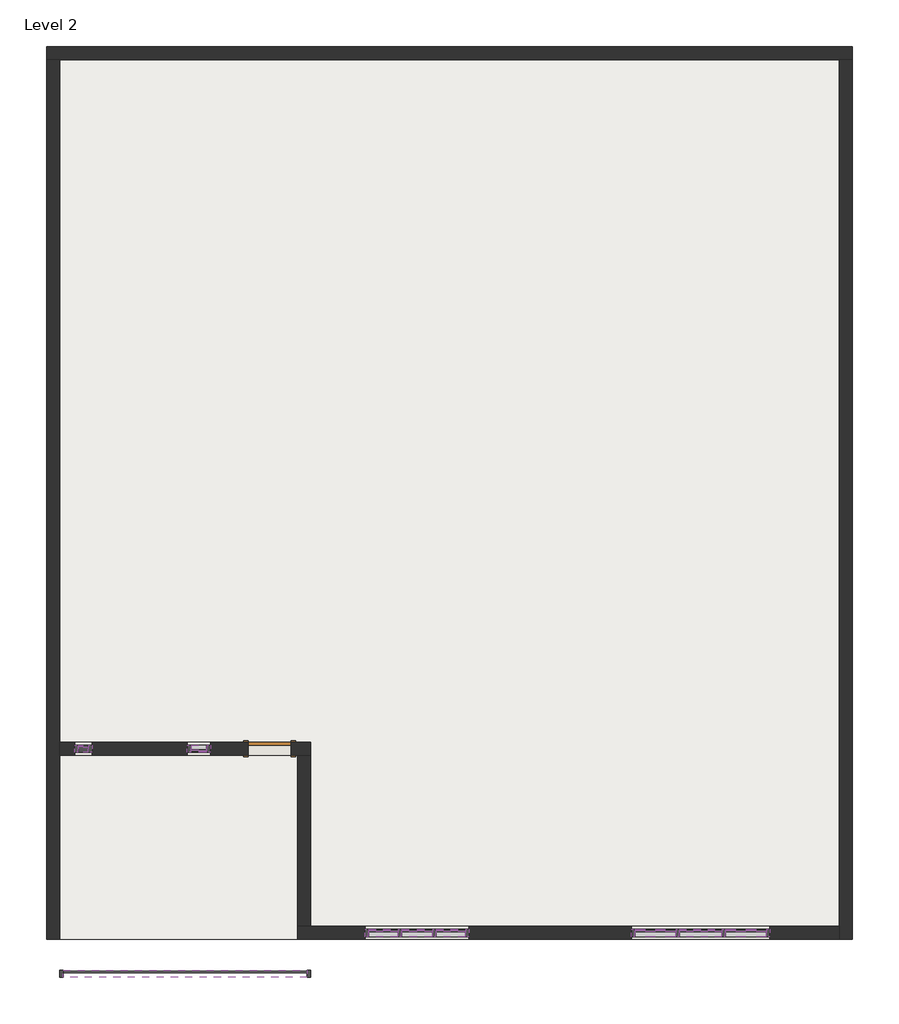
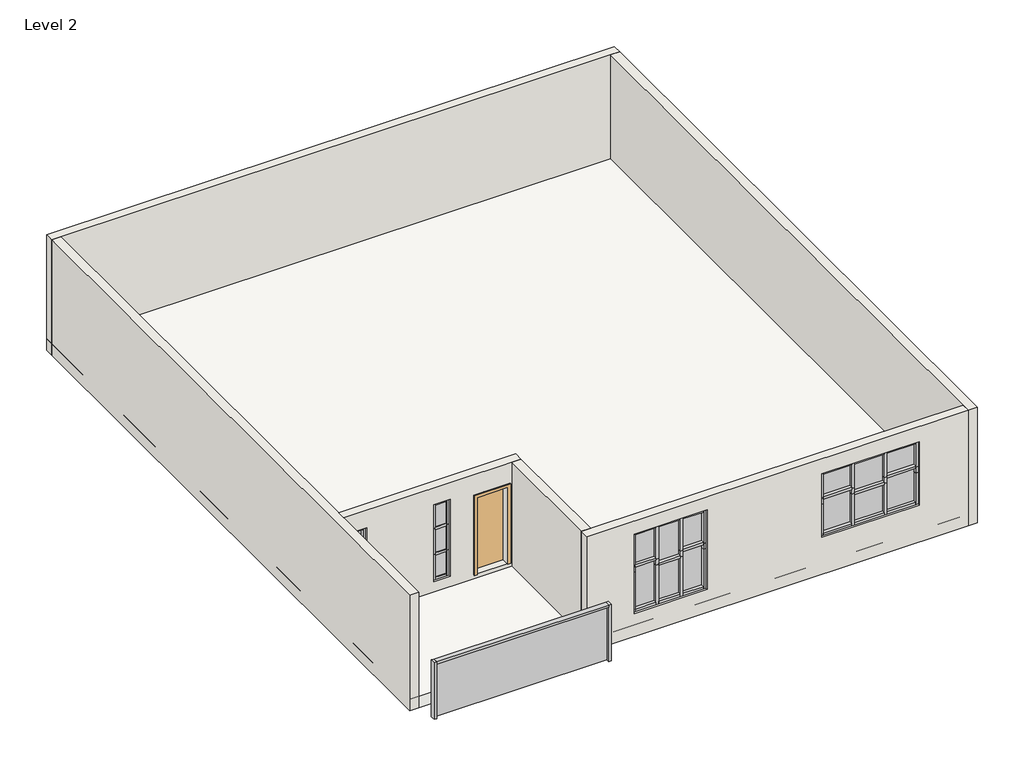
# One storey: 65 members, 19 plates, 6 walls, 1 door, 1 roof.
"""IFC4 building model written with IfcOpenShell, lengths in millimetres."""

from ifc_helpers import new_model, si_unit, frame, origin, place, context, project, spatial, polyline, outline, extrude, faceted_brep, transform, mapped, element, save
from components import door_a1484949, member_aaa03826, member_0b7646a3, member_a980948f, member_0a1a1ade, member_876f8f00, member_f6f0dfdd, member_50c8646f, member_e2125230, member_501daf10, member_2a6e7b3e, member_892f3d40, member_7007ad49, member_abeaf8ac, member_2c92067c, member_9d02be77, member_798d6cad, member_1bc815af, member_262c5f3f, member_6be37683, member_d3323a85, member_819a76f2, member_187b6476, member_d92184fb, member_2118ea0c, member_241584b0, member_4da692ab, system_panel_glazed_51e75bbe, system_panel_glazed_29e6fa37, system_panel_glazed_a0a4d195, system_panel_glazed_09326d9e, system_panel_glazed_ba8d0b35, system_panel_glazed_02566968, system_panel_glazed_4b08eeb4, system_panel_glazed_a2941881, system_panel_glazed_2307425d, system_panel_glazed_f1f3e2b8, system_panel_glazed_c39d0069, system_panel_glazed_879596d7, system_panel_glazed_4ec28fe5

model = new_model("IFC4")

# Units and contexts
model_context = context("Model", 3, world=origin())
ifc_project = project(units=[si_unit("LENGTHUNIT", "METRE", prefix="MILLI")], contexts=[model_context])

# Site, building, storey
site = spatial("IfcSite", under=ifc_project)
building = spatial("IfcBuilding", under=site)
storey = spatial("IfcBuildingStorey", under=building, Name="Level 2", Elevation=3048.0)

# Door
placement = place(None, origin())
door_shape = door_a1484949(model_context)
element("IfcDoor", 1, ObjectType="Single-Flush : 30\" x 80\"", at=placement, inside=storey, context=model_context, shape_type="MappedRepresentation", body=[
    mapped(door_shape, transform((-15264.8403308, -10002.5518738, 3454.4), x_axis=(1.0, 0.0, 0.0), y_axis=(0.0, 1.0, 0.0), z_axis=(0.0, 0.0, 1.0))),
])

# Members
member_shape = member_aaa03826(model_context)
element("IfcMember", 2, ObjectType="Rectangular Mullion : 2.5\" x 5\" rectangular", at=placement, inside=storey, context=model_context, shape_type="MappedRepresentation", body=[
    mapped(member_shape, transform((-11823.1403308, -13241.0518738, 4852.5078277), x_axis=(0.0, 0.0, 1.0), y_axis=(0.0, -1.0, 0.0), z_axis=(1.0, 0.0, 0.0))),
])
element("IfcMember", 3, ObjectType="Rectangular Mullion : 2.5\" x 5\" rectangular", at=placement, inside=storey, context=model_context, shape_type="MappedRepresentation", body=[
    mapped(member_shape, transform((-13010.5903308, -13241.0518738, 4852.5078277), x_axis=(0.0, 0.0, 1.0), y_axis=(0.0, -1.0, 0.0), z_axis=(1.0, 0.0, 0.0))),
])
member_2_shape = member_0b7646a3(model_context)
element("IfcMember", 4, ObjectType="Rectangular Mullion : 2.5\" x 5\" rectangular", at=placement, inside=storey, context=model_context, shape_type="MappedRepresentation", body=[
    mapped(member_2_shape, transform((-13010.5903308, -13241.0518738, 5747.4569224), x_axis=(0.0, 0.0, 1.0), y_axis=(0.0, -1.0, 0.0), z_axis=(1.0, 0.0, 0.0))),
])
element("IfcMember", 5, ObjectType="Rectangular Mullion : 2.5\" x 5\" rectangular", at=placement, inside=storey, context=model_context, shape_type="MappedRepresentation", body=[
    mapped(member_2_shape, transform((-11823.1403308, -13241.0518738, 5747.4569224), x_axis=(0.0, 0.0, 1.0), y_axis=(0.0, -1.0, 0.0), z_axis=(1.0, 0.0, 0.0))),
])
member_3_shape = member_a980948f(model_context)
element("IfcMember", 6, ObjectType="Rectangular Mullion : 2.5\" x 5\" rectangular", at=placement, inside=storey, context=model_context, shape_type="MappedRepresentation", body=[
    mapped(member_3_shape, transform((-12400.9903308, -13241.0518738, 5747.4569224), x_axis=(0.0, 0.0, 1.0), y_axis=(0.0, -1.0, 0.0), z_axis=(1.0, 0.0, 0.0))),
])
member_4_shape = member_0a1a1ade(model_context)
element("IfcMember", 7, ObjectType="Rectangular Mullion : 2.5\" x 5\" rectangular", at=placement, inside=storey, context=model_context, shape_type="MappedRepresentation", body=[
    mapped(member_4_shape, transform((-12400.9903308, -13241.0518738, 4700.1078277), x_axis=(0.0, 0.0, 1.0), y_axis=(0.0, -1.0, 0.0), z_axis=(1.0, 0.0, 0.0))),
])
element("IfcMember", 8, ObjectType="Rectangular Mullion : 2.5\" x 5\" rectangular", at=placement, inside=storey, context=model_context, shape_type="MappedRepresentation", body=[
    mapped(member_2_shape, transform((-12337.4903308, -13241.0518738, 3652.758733), x_axis=(0.0, 0.0, -1.0), y_axis=(0.0, -1.0, 0.0), z_axis=(-1.0, 0.0, 0.0))),
])
element("IfcMember", 9, ObjectType="Rectangular Mullion : 2.5\" x 5\" rectangular", at=placement, inside=storey, context=model_context, shape_type="MappedRepresentation", body=[
    mapped(member_2_shape, transform((-13524.9403308, -13241.0518738, 3652.758733), x_axis=(0.0, 0.0, -1.0), y_axis=(0.0, -1.0, 0.0), z_axis=(-1.0, 0.0, 0.0))),
])
element("IfcMember", 10, ObjectType="Rectangular Mullion : 2.5\" x 5\" rectangular", at=placement, inside=storey, context=model_context, shape_type="MappedRepresentation", body=[
    mapped(member_3_shape, transform((-12947.0903308, -13241.0518738, 3652.758733), x_axis=(0.0, 0.0, -1.0), y_axis=(0.0, -1.0, 0.0), z_axis=(-1.0, 0.0, 0.0))),
])
member_5_shape = member_876f8f00(model_context)
element("IfcMember", 11, ObjectType="Rectangular Mullion : 2.5\" x 5\" rectangular", at=placement, inside=storey, context=model_context, shape_type="MappedRepresentation", body=[
    mapped(member_5_shape, transform((-13588.4403308, -13241.0518738, 4852.5078277), x_axis=(-1.0, 0.0, 0.0), y_axis=(0.0, -1.0, 0.0), z_axis=(0.0, 0.0, 1.0))),
])
element("IfcMember", 12, ObjectType="Rectangular Mullion : 2.5\" x 5\" rectangular", at=placement, inside=storey, context=model_context, shape_type="MappedRepresentation", body=[
    mapped(member_5_shape, transform((-8902.1403308, -13241.0518738, 5010.2067568), x_axis=(-1.0, 0.0, 0.0), y_axis=(0.0, -1.0, 0.0), z_axis=(0.0, 0.0, 1.0))),
])
element("IfcMember", 13, ObjectType="Rectangular Mullion : 2.5\" x 5\" rectangular", at=placement, inside=storey, context=model_context, shape_type="MappedRepresentation", body=[
    mapped(member_5_shape, transform((-11759.6403308, -13241.0518738, 4700.1078277), x_axis=(1.0, 0.0, 0.0), y_axis=(0.0, -1.0, 0.0), z_axis=(0.0, 0.0, -1.0))),
])
element("IfcMember", 14, ObjectType="Rectangular Mullion : 2.5\" x 5\" rectangular", at=placement, inside=storey, context=model_context, shape_type="MappedRepresentation", body=[
    mapped(member_5_shape, transform((-6463.7403308, -13241.0518738, 4857.8067568), x_axis=(1.0, 0.0, 0.0), y_axis=(0.0, -1.0, 0.0), z_axis=(0.0, 0.0, -1.0))),
])
member_6_shape = member_f6f0dfdd(model_context)
element("IfcMember", 15, ObjectType="Rectangular Mullion : 2.5\" x 5\" rectangular", at=placement, inside=storey, context=model_context, shape_type="MappedRepresentation", body=[
    mapped(member_6_shape, transform((-12978.8403308, -13241.0518738, 4700.1078277), x_axis=(1.0, 0.0, 0.0), y_axis=(0.0, -1.0, 0.0), z_axis=(0.0, 0.0, -1.0))),
])
element("IfcMember", 16, ObjectType="Rectangular Mullion : 2.5\" x 5\" rectangular", at=placement, inside=storey, context=model_context, shape_type="MappedRepresentation", body=[
    mapped(member_6_shape, transform((-12369.2403308, -13241.0518738, 4700.1078277), x_axis=(1.0, 0.0, 0.0), y_axis=(0.0, -1.0, 0.0), z_axis=(0.0, 0.0, -1.0))),
])
element("IfcMember", 17, ObjectType="Rectangular Mullion : 2.5\" x 5\" rectangular", at=placement, inside=storey, context=model_context, shape_type="MappedRepresentation", body=[
    mapped(member_6_shape, transform((-8089.3403308, -13241.0518738, 4857.8067568), x_axis=(1.0, 0.0, 0.0), y_axis=(0.0, -1.0, 0.0), z_axis=(0.0, 0.0, -1.0))),
])
element("IfcMember", 18, ObjectType="Rectangular Mullion : 2.5\" x 5\" rectangular", at=placement, inside=storey, context=model_context, shape_type="MappedRepresentation", body=[
    mapped(member_6_shape, transform((-7276.5403308, -13241.0518738, 4857.8067568), x_axis=(1.0, 0.0, 0.0), y_axis=(0.0, -1.0, 0.0), z_axis=(0.0, 0.0, -1.0))),
])
member_7_shape = member_50c8646f(model_context)
element("IfcMember", 19, ObjectType="Rectangular Mullion : 2.5\" x 5\" rectangular", at=placement, inside=storey, context=model_context, shape_type="MappedRepresentation", body=[
    mapped(member_7_shape, transform((-12978.8403308, -13241.0518738, 4852.5078277), x_axis=(1.0, 0.0, 0.0), y_axis=(0.0, -1.0, 0.0), z_axis=(0.0, 0.0, -1.0))),
])
element("IfcMember", 20, ObjectType="Rectangular Mullion : 2.5\" x 5\" rectangular", at=placement, inside=storey, context=model_context, shape_type="MappedRepresentation", body=[
    mapped(member_7_shape, transform((-12369.2403308, -13241.0518738, 4852.5078277), x_axis=(1.0, 0.0, 0.0), y_axis=(0.0, -1.0, 0.0), z_axis=(0.0, 0.0, -1.0))),
])
member_8_shape = member_e2125230(model_context)
element("IfcMember", 21, ObjectType="Rectangular Mullion : 2.5\" x 5\" rectangular", at=placement, inside=storey, context=model_context, shape_type="MappedRepresentation", body=[
    mapped(member_8_shape, transform((-11759.6403308, -13241.0518738, 4852.5078277), x_axis=(1.0, 0.0, 0.0), y_axis=(0.0, -1.0, 0.0), z_axis=(0.0, 0.0, -1.0))),
])
element("IfcMember", 22, ObjectType="Rectangular Mullion : 2.5\" x 5\" rectangular", at=placement, inside=storey, context=model_context, shape_type="MappedRepresentation", body=[
    mapped(member_8_shape, transform((-13588.4403308, -13241.0518738, 5747.4569224), x_axis=(-1.0, 0.0, 0.0), y_axis=(0.0, -1.0, 0.0), z_axis=(0.0, 0.0, 1.0))),
])
member_9_shape = member_501daf10(model_context)
element("IfcMember", 23, ObjectType="Rectangular Mullion : 2.5\" x 5\" rectangular", at=placement, inside=storey, context=model_context, shape_type="MappedRepresentation", body=[
    mapped(member_9_shape, transform((-12978.8403308, -13241.0518738, 3652.758733), x_axis=(1.0, 0.0, 0.0), y_axis=(0.0, -1.0, 0.0), z_axis=(0.0, 0.0, -1.0))),
])
element("IfcMember", 24, ObjectType="Rectangular Mullion : 2.5\" x 5\" rectangular", at=placement, inside=storey, context=model_context, shape_type="MappedRepresentation", body=[
    mapped(member_9_shape, transform((-12369.2403308, -13241.0518738, 3652.758733), x_axis=(1.0, 0.0, 0.0), y_axis=(0.0, -1.0, 0.0), z_axis=(0.0, 0.0, -1.0))),
])
member_10_shape = member_2a6e7b3e(model_context)
element("IfcMember", 25, ObjectType="Rectangular Mullion : 2.5\" x 5\" rectangular", at=placement, inside=storey, context=model_context, shape_type="MappedRepresentation", body=[
    mapped(member_10_shape, transform((-11759.6403308, -13241.0518738, 3652.758733), x_axis=(1.0, 0.0, 0.0), y_axis=(0.0, -1.0, 0.0), z_axis=(0.0, 0.0, -1.0))),
])
element("IfcMember", 26, ObjectType="Rectangular Mullion : 2.5\" x 5\" rectangular", at=placement, inside=storey, context=model_context, shape_type="MappedRepresentation", body=[
    mapped(member_10_shape, transform((-13588.4403308, -13241.0518738, 4700.1078277), x_axis=(-1.0, 0.0, 0.0), y_axis=(0.0, -1.0, 0.0), z_axis=(0.0, 0.0, 1.0))),
])
member_11_shape = member_892f3d40(model_context)
element("IfcMember", 27, ObjectType="Rectangular Mullion : 2.5\" x 5\" rectangular", at=placement, inside=storey, context=model_context, shape_type="MappedRepresentation", body=[
    mapped(member_11_shape, transform((-8902.1403308, -13241.0518738, 5695.6642445), x_axis=(-1.0, 0.0, 0.0), y_axis=(0.0, -1.0, 0.0), z_axis=(0.0, 0.0, 1.0))),
])
member_12_shape = member_7007ad49(model_context)
element("IfcMember", 28, ObjectType="Rectangular Mullion : 2.5\" x 5\" rectangular", at=placement, inside=storey, context=model_context, shape_type="MappedRepresentation", body=[
    mapped(member_12_shape, transform((-8121.0903308, -13241.0518738, 5695.6642445), x_axis=(0.0, 0.0, 1.0), y_axis=(0.0, -1.0, 0.0), z_axis=(1.0, 0.0, 0.0))),
])
element("IfcMember", 29, ObjectType="Rectangular Mullion : 2.5\" x 5\" rectangular", at=placement, inside=storey, context=model_context, shape_type="MappedRepresentation", body=[
    mapped(member_12_shape, transform((-6527.2403308, -13241.0518738, 5695.6642445), x_axis=(0.0, 0.0, 1.0), y_axis=(0.0, -1.0, 0.0), z_axis=(1.0, 0.0, 0.0))),
])
member_13_shape = member_abeaf8ac(model_context)
element("IfcMember", 30, ObjectType="Rectangular Mullion : 2.5\" x 5\" rectangular", at=placement, inside=storey, context=model_context, shape_type="MappedRepresentation", body=[
    mapped(member_13_shape, transform((-6527.2403308, -13241.0518738, 5010.2067568), x_axis=(0.0, 0.0, 1.0), y_axis=(0.0, -1.0, 0.0), z_axis=(1.0, 0.0, 0.0))),
])
element("IfcMember", 31, ObjectType="Rectangular Mullion : 2.5\" x 5\" rectangular", at=placement, inside=storey, context=model_context, shape_type="MappedRepresentation", body=[
    mapped(member_13_shape, transform((-8121.0903308, -13241.0518738, 5010.2067568), x_axis=(0.0, 0.0, 1.0), y_axis=(0.0, -1.0, 0.0), z_axis=(1.0, 0.0, 0.0))),
])
member_14_shape = member_2c92067c(model_context)
element("IfcMember", 32, ObjectType="Rectangular Mullion : 2.5\" x 5\" rectangular", at=placement, inside=storey, context=model_context, shape_type="MappedRepresentation", body=[
    mapped(member_14_shape, transform((-8089.3403308, -13241.0518738, 5010.2067568), x_axis=(1.0, 0.0, 0.0), y_axis=(0.0, -1.0, 0.0), z_axis=(0.0, 0.0, -1.0))),
])
element("IfcMember", 33, ObjectType="Rectangular Mullion : 2.5\" x 5\" rectangular", at=placement, inside=storey, context=model_context, shape_type="MappedRepresentation", body=[
    mapped(member_14_shape, transform((-7276.5403308, -13241.0518738, 5010.2067568), x_axis=(1.0, 0.0, 0.0), y_axis=(0.0, -1.0, 0.0), z_axis=(0.0, 0.0, -1.0))),
])
member_15_shape = member_9d02be77(model_context)
element("IfcMember", 34, ObjectType="Rectangular Mullion : 2.5\" x 5\" rectangular", at=placement, inside=storey, context=model_context, shape_type="MappedRepresentation", body=[
    mapped(member_15_shape, transform((-7308.2903308, -13241.0518738, 5695.6642445), x_axis=(0.0, 0.0, 1.0), y_axis=(0.0, -1.0, 0.0), z_axis=(1.0, 0.0, 0.0))),
])
member_16_shape = member_798d6cad(model_context)
element("IfcMember", 35, ObjectType="Rectangular Mullion : 2.5\" x 5\" rectangular", at=placement, inside=storey, context=model_context, shape_type="MappedRepresentation", body=[
    mapped(member_16_shape, transform((-7308.2903308, -13241.0518738, 4857.8067568), x_axis=(0.0, 0.0, 1.0), y_axis=(0.0, -1.0, 0.0), z_axis=(1.0, 0.0, 0.0))),
])
element("IfcMember", 36, ObjectType="Rectangular Mullion : 2.5\" x 5\" rectangular", at=placement, inside=storey, context=model_context, shape_type="MappedRepresentation", body=[
    mapped(member_11_shape, transform((-6463.7403308, -13241.0518738, 5010.2067568), x_axis=(1.0, 0.0, 0.0), y_axis=(0.0, -1.0, 0.0), z_axis=(0.0, 0.0, -1.0))),
])
member_17_shape = member_1bc815af(model_context)
element("IfcMember", 37, ObjectType="Rectangular Mullion : 2.5\" x 5\" rectangular", at=placement, inside=storey, context=model_context, shape_type="MappedRepresentation", body=[
    mapped(member_17_shape, transform((-8089.3403308, -13241.0518738, 4019.949269), x_axis=(1.0, 0.0, 0.0), y_axis=(0.0, -1.0, 0.0), z_axis=(0.0, 0.0, -1.0))),
])
element("IfcMember", 38, ObjectType="Rectangular Mullion : 2.5\" x 5\" rectangular", at=placement, inside=storey, context=model_context, shape_type="MappedRepresentation", body=[
    mapped(member_17_shape, transform((-7276.5403308, -13241.0518738, 4019.949269), x_axis=(1.0, 0.0, 0.0), y_axis=(0.0, -1.0, 0.0), z_axis=(0.0, 0.0, -1.0))),
])
element("IfcMember", 39, ObjectType="Rectangular Mullion : 2.5\" x 5\" rectangular", at=placement, inside=storey, context=model_context, shape_type="MappedRepresentation", body=[
    mapped(member_12_shape, transform((-7244.7903308, -13241.0518738, 4019.949269), x_axis=(0.0, 0.0, -1.0), y_axis=(0.0, -1.0, 0.0), z_axis=(-1.0, 0.0, 0.0))),
])
element("IfcMember", 40, ObjectType="Rectangular Mullion : 2.5\" x 5\" rectangular", at=placement, inside=storey, context=model_context, shape_type="MappedRepresentation", body=[
    mapped(member_12_shape, transform((-8838.6403308, -13241.0518738, 4019.949269), x_axis=(0.0, 0.0, -1.0), y_axis=(0.0, -1.0, 0.0), z_axis=(-1.0, 0.0, 0.0))),
])
element("IfcMember", 41, ObjectType="Rectangular Mullion : 2.5\" x 5\" rectangular", at=placement, inside=storey, context=model_context, shape_type="MappedRepresentation", body=[
    mapped(member_15_shape, transform((-8057.5903308, -13241.0518738, 4019.949269), x_axis=(0.0, 0.0, -1.0), y_axis=(0.0, -1.0, 0.0), z_axis=(-1.0, 0.0, 0.0))),
])
member_18_shape = member_262c5f3f(model_context)
element("IfcMember", 42, ObjectType="Rectangular Mullion : 2.5\" x 5\" rectangular", at=placement, inside=storey, context=model_context, shape_type="MappedRepresentation", body=[
    mapped(member_18_shape, transform((-8902.1403308, -13241.0518738, 4857.8067568), x_axis=(-1.0, 0.0, 0.0), y_axis=(0.0, -1.0, 0.0), z_axis=(0.0, 0.0, 1.0))),
])
element("IfcMember", 43, ObjectType="Rectangular Mullion : 2.5\" x 5\" rectangular", at=placement, inside=storey, context=model_context, shape_type="MappedRepresentation", body=[
    mapped(member_18_shape, transform((-6463.7403308, -13241.0518738, 4019.949269), x_axis=(1.0, 0.0, 0.0), y_axis=(0.0, -1.0, 0.0), z_axis=(0.0, 0.0, -1.0))),
])
member_19_shape = member_6be37683(model_context)
element("IfcMember", 44, ObjectType="Rectangular Mullion : 2.5\" x 5\" rectangular", at=placement, inside=storey, context=model_context, shape_type="MappedRepresentation", body=[
    mapped(member_19_shape, transform((-16649.1403308, -10002.5518738, 4978.7509018), x_axis=(0.0, 0.0, 1.0), y_axis=(0.0, 1.0, 0.0), z_axis=(-1.0, 0.0, 0.0))),
])
element("IfcMember", 45, ObjectType="Rectangular Mullion : 2.5\" x 5\" rectangular", at=placement, inside=storey, context=model_context, shape_type="MappedRepresentation", body=[
    mapped(member_19_shape, transform((-16649.1403308, -10002.5518738, 4301.7310778), x_axis=(0.0, 0.0, 1.0), y_axis=(0.0, 1.0, 0.0), z_axis=(-1.0, 0.0, 0.0))),
])
member_20_shape = member_d3323a85(model_context)
element("IfcMember", 46, ObjectType="Rectangular Mullion : 2.5\" x 5\" rectangular", at=placement, inside=storey, context=model_context, shape_type="MappedRepresentation", body=[
    mapped(member_20_shape, transform((-16649.1403308, -10002.5518738, 5655.7707259), x_axis=(0.0, 0.0, 1.0), y_axis=(0.0, 1.0, 0.0), z_axis=(-1.0, 0.0, 0.0))),
])
member_21_shape = member_819a76f2(model_context)
element("IfcMember", 47, ObjectType="Rectangular Mullion : 2.5\" x 5\" rectangular", at=placement, inside=storey, context=model_context, shape_type="MappedRepresentation", body=[
    mapped(member_21_shape, transform((-16712.6403308, -10002.5518738, 4978.7509018), x_axis=(-1.0, 0.0, 0.0), y_axis=(0.0, 1.0, 0.0), z_axis=(0.0, 0.0, -1.0))),
])
element("IfcMember", 48, ObjectType="Rectangular Mullion : 2.5\" x 5\" rectangular", at=placement, inside=storey, context=model_context, shape_type="MappedRepresentation", body=[
    mapped(member_21_shape, transform((-16306.2403308, -10002.5518738, 5655.7707259), x_axis=(1.0, 0.0, 0.0), y_axis=(0.0, 1.0, 0.0), z_axis=(0.0, 0.0, 1.0))),
])
element("IfcMember", 49, ObjectType="Rectangular Mullion : 2.5\" x 5\" rectangular", at=placement, inside=storey, context=model_context, shape_type="MappedRepresentation", body=[
    mapped(member_21_shape, transform((-16712.6403308, -10002.5518738, 4301.7310778), x_axis=(-1.0, 0.0, 0.0), y_axis=(0.0, 1.0, 0.0), z_axis=(0.0, 0.0, -1.0))),
])
element("IfcMember", 50, ObjectType="Rectangular Mullion : 2.5\" x 5\" rectangular", at=placement, inside=storey, context=model_context, shape_type="MappedRepresentation", body=[
    mapped(member_21_shape, transform((-16306.2403308, -10002.5518738, 4978.7509018), x_axis=(1.0, 0.0, 0.0), y_axis=(0.0, 1.0, 0.0), z_axis=(0.0, 0.0, 1.0))),
])
element("IfcMember", 51, ObjectType="Rectangular Mullion : 2.5\" x 5\" rectangular", at=placement, inside=storey, context=model_context, shape_type="MappedRepresentation", body=[
    mapped(member_20_shape, transform((-16369.7403308, -10002.5518738, 3624.7112538), x_axis=(0.0, 0.0, -1.0), y_axis=(0.0, 1.0, 0.0), z_axis=(1.0, 0.0, 0.0))),
])
element("IfcMember", 52, ObjectType="Rectangular Mullion : 2.5\" x 5\" rectangular", at=placement, inside=storey, context=model_context, shape_type="MappedRepresentation", body=[
    mapped(member_21_shape, transform((-16712.6403308, -10002.5518738, 3624.7112538), x_axis=(-1.0, 0.0, 0.0), y_axis=(0.0, 1.0, 0.0), z_axis=(0.0, 0.0, -1.0))),
])
element("IfcMember", 53, ObjectType="Rectangular Mullion : 2.5\" x 5\" rectangular", at=placement, inside=storey, context=model_context, shape_type="MappedRepresentation", body=[
    mapped(member_21_shape, transform((-16306.2403308, -10002.5518738, 4301.7310778), x_axis=(1.0, 0.0, 0.0), y_axis=(0.0, 1.0, 0.0), z_axis=(0.0, 0.0, 1.0))),
])
member_22_shape = member_187b6476(model_context)
element("IfcMember", 54, ObjectType="Rectangular Mullion : 2.5\" x 5\" rectangular", at=placement, inside=storey, context=model_context, shape_type="MappedRepresentation", body=[
    mapped(member_22_shape, transform((-18389.0403308, -10002.5518738, 4957.2410097), x_axis=(1.0, 0.0, 0.0), y_axis=(0.0, -1.0, 0.0), z_axis=(0.0, 0.0, -1.0))),
])
member_23_shape = member_d92184fb(model_context)
element("IfcMember", 55, ObjectType="Rectangular Mullion : 2.5\" x 5\" rectangular", at=placement, inside=storey, context=model_context, shape_type="MappedRepresentation", body=[
    mapped(member_23_shape, transform((-18452.5403308, -10002.5518738, 5641.0036022), x_axis=(0.0, 0.0, 1.0), y_axis=(0.0, -1.0, 0.0), z_axis=(1.0, 0.0, 0.0))),
])
member_24_shape = member_2118ea0c(model_context)
element("IfcMember", 56, ObjectType="Rectangular Mullion : 2.5\" x 5\" rectangular", at=placement, inside=storey, context=model_context, shape_type="MappedRepresentation", body=[
    mapped(member_24_shape, transform((-18452.5403308, -10002.5518738, 4957.2410097), x_axis=(0.0, 0.0, 1.0), y_axis=(0.0, -1.0, 0.0), z_axis=(1.0, 0.0, 0.0))),
])
element("IfcMember", 57, ObjectType="Rectangular Mullion : 2.5\" x 5\" rectangular", at=placement, inside=storey, context=model_context, shape_type="MappedRepresentation", body=[
    mapped(member_24_shape, transform((-18452.5403308, -10002.5518738, 4273.4784172), x_axis=(0.0, 0.0, 1.0), y_axis=(0.0, -1.0, 0.0), z_axis=(1.0, 0.0, 0.0))),
])
element("IfcMember", 58, ObjectType="Rectangular Mullion : 2.5\" x 5\" rectangular", at=placement, inside=storey, context=model_context, shape_type="MappedRepresentation", body=[
    mapped(member_22_shape, transform((-18693.8403308, -10002.5518738, 5641.0036022), x_axis=(-1.0, 0.0, 0.0), y_axis=(0.0, -1.0, 0.0), z_axis=(0.0, 0.0, 1.0))),
])
element("IfcMember", 59, ObjectType="Rectangular Mullion : 2.5\" x 5\" rectangular", at=placement, inside=storey, context=model_context, shape_type="MappedRepresentation", body=[
    mapped(member_22_shape, transform((-18389.0403308, -10002.5518738, 4273.4784172), x_axis=(1.0, 0.0, 0.0), y_axis=(0.0, -1.0, 0.0), z_axis=(0.0, 0.0, -1.0))),
])
element("IfcMember", 60, ObjectType="Rectangular Mullion : 2.5\" x 5\" rectangular", at=placement, inside=storey, context=model_context, shape_type="MappedRepresentation", body=[
    mapped(member_22_shape, transform((-18693.8403308, -10002.5518738, 4957.2410097), x_axis=(-1.0, 0.0, 0.0), y_axis=(0.0, -1.0, 0.0), z_axis=(0.0, 0.0, 1.0))),
])
element("IfcMember", 61, ObjectType="Rectangular Mullion : 2.5\" x 5\" rectangular", at=placement, inside=storey, context=model_context, shape_type="MappedRepresentation", body=[
    mapped(member_23_shape, transform((-18630.3403308, -10002.5518738, 3589.7158247), x_axis=(0.0, 0.0, -1.0), y_axis=(0.0, -1.0, 0.0), z_axis=(-1.0, 0.0, 0.0))),
])
element("IfcMember", 62, ObjectType="Rectangular Mullion : 2.5\" x 5\" rectangular", at=placement, inside=storey, context=model_context, shape_type="MappedRepresentation", body=[
    mapped(member_22_shape, transform((-18389.0403308, -10002.5518738, 3589.7158247), x_axis=(1.0, 0.0, 0.0), y_axis=(0.0, -1.0, 0.0), z_axis=(0.0, 0.0, -1.0))),
])
element("IfcMember", 63, ObjectType="Rectangular Mullion : 2.5\" x 5\" rectangular", at=placement, inside=storey, context=model_context, shape_type="MappedRepresentation", body=[
    mapped(member_22_shape, transform((-18693.8403308, -10002.5518738, 4273.4784172), x_axis=(-1.0, 0.0, 0.0), y_axis=(0.0, -1.0, 0.0), z_axis=(0.0, 0.0, 1.0))),
])
member_25_shape = member_241584b0(model_context)
element("IfcMember", 64, ObjectType="Rectangular Mullion : 2.5\" x 5\" rectangular", at=placement, inside=storey, context=model_context, shape_type="MappedRepresentation", body=[
    mapped(member_25_shape, transform((-18960.5403308, -13959.4936073, 4638.740692), x_axis=(-1.0, 0.0, 0.0), y_axis=(0.0, -1.0, 0.0), z_axis=(0.0, 0.0, 1.0))),
])
member_26_shape = member_4da692ab(model_context)
element("IfcMember", 65, ObjectType="Rectangular Mullion : 2.5\" x 5\" rectangular", at=placement, inside=storey, context=model_context, shape_type="MappedRepresentation", body=[
    mapped(member_26_shape, transform((-14604.4403308, -13959.4936073, 4638.740692), x_axis=(0.0, 0.0, 1.0), y_axis=(0.0, -1.0, 0.0), z_axis=(1.0, 0.0, 0.0))),
])
element("IfcMember", 66, ObjectType="Rectangular Mullion : 2.5\" x 5\" rectangular", at=placement, inside=storey, context=model_context, shape_type="MappedRepresentation", body=[
    mapped(member_25_shape, transform((-14540.9403308, -13959.4936073, 3145.1973892), x_axis=(1.0, 0.0, 0.0), y_axis=(0.0, -1.0, 0.0), z_axis=(0.0, 0.0, -1.0))),
])

# Plates
system_panel_glazed_shape = system_panel_glazed_51e75bbe(model_context)
element("IfcPlate", 67, ObjectType="System Panel : Glazed", at=placement, inside=storey, context=model_context, shape_type="MappedRepresentation", body=[
    mapped(system_panel_glazed_shape, transform((-12674.0403308, -13241.0518738, 4731.8578277), x_axis=(1.0, 0.0, 0.0), y_axis=(0.0, 1.0, 0.0), z_axis=(0.0, 0.0, 1.0))),
])
system_panel_glazed_2_shape = system_panel_glazed_29e6fa37(model_context)
element("IfcPlate", 68, ObjectType="System Panel : Glazed", at=placement, inside=storey, context=model_context, shape_type="MappedRepresentation", body=[
    mapped(system_panel_glazed_2_shape, transform((-13267.7653308, -13241.0518738, 4884.2578277), x_axis=(1.0, 0.0, 0.0), y_axis=(0.0, 1.0, 0.0), z_axis=(0.0, 0.0, 1.0))),
])
element("IfcPlate", 69, ObjectType="System Panel : Glazed", at=placement, inside=storey, context=model_context, shape_type="MappedRepresentation", body=[
    mapped(system_panel_glazed_2_shape, transform((-12080.3153308, -13241.0518738, 4884.2578277), x_axis=(1.0, 0.0, 0.0), y_axis=(0.0, 1.0, 0.0), z_axis=(0.0, 0.0, 1.0))),
])
system_panel_glazed_3_shape = system_panel_glazed_a0a4d195(model_context)
element("IfcPlate", 70, ObjectType="System Panel : Glazed", at=placement, inside=storey, context=model_context, shape_type="MappedRepresentation", body=[
    mapped(system_panel_glazed_3_shape, transform((-13267.7653308, -13241.0518738, 3716.258733), x_axis=(1.0, 0.0, 0.0), y_axis=(0.0, 1.0, 0.0), z_axis=(0.0, 0.0, 1.0))),
])
element("IfcPlate", 71, ObjectType="System Panel : Glazed", at=placement, inside=storey, context=model_context, shape_type="MappedRepresentation", body=[
    mapped(system_panel_glazed_3_shape, transform((-12080.3153308, -13241.0518738, 3716.258733), x_axis=(1.0, 0.0, 0.0), y_axis=(0.0, 1.0, 0.0), z_axis=(0.0, 0.0, 1.0))),
])
system_panel_glazed_4_shape = system_panel_glazed_09326d9e(model_context)
element("IfcPlate", 72, ObjectType="System Panel : Glazed", at=placement, inside=storey, context=model_context, shape_type="MappedRepresentation", body=[
    mapped(system_panel_glazed_4_shape, transform((-12674.0403308, -13241.0518738, 3716.258733), x_axis=(1.0, 0.0, 0.0), y_axis=(0.0, 1.0, 0.0), z_axis=(0.0, 0.0, 1.0))),
])
system_panel_glazed_5_shape = system_panel_glazed_ba8d0b35(model_context)
element("IfcPlate", 73, ObjectType="System Panel : Glazed", at=placement, inside=storey, context=model_context, shape_type="MappedRepresentation", body=[
    mapped(system_panel_glazed_5_shape, transform((-8479.8653308, -13241.0518738, 5041.9567568), x_axis=(1.0, 0.0, 0.0), y_axis=(0.0, 1.0, 0.0), z_axis=(0.0, 0.0, 1.0))),
])
element("IfcPlate", 74, ObjectType="System Panel : Glazed", at=placement, inside=storey, context=model_context, shape_type="MappedRepresentation", body=[
    mapped(system_panel_glazed_5_shape, transform((-6886.0153308, -13241.0518738, 5041.9567568), x_axis=(1.0, 0.0, 0.0), y_axis=(0.0, 1.0, 0.0), z_axis=(0.0, 0.0, 1.0))),
])
system_panel_glazed_6_shape = system_panel_glazed_02566968(model_context)
element("IfcPlate", 75, ObjectType="System Panel : Glazed", at=placement, inside=storey, context=model_context, shape_type="MappedRepresentation", body=[
    mapped(system_panel_glazed_6_shape, transform((-7682.9403308, -13241.0518738, 4889.5567568), x_axis=(1.0, 0.0, 0.0), y_axis=(0.0, 1.0, 0.0), z_axis=(0.0, 0.0, 1.0))),
])
system_panel_glazed_7_shape = system_panel_glazed_4b08eeb4(model_context)
element("IfcPlate", 76, ObjectType="System Panel : Glazed", at=placement, inside=storey, context=model_context, shape_type="MappedRepresentation", body=[
    mapped(system_panel_glazed_7_shape, transform((-8479.8653308, -13241.0518738, 4083.449269), x_axis=(1.0, 0.0, 0.0), y_axis=(0.0, 1.0, 0.0), z_axis=(0.0, 0.0, 1.0))),
])
element("IfcPlate", 77, ObjectType="System Panel : Glazed", at=placement, inside=storey, context=model_context, shape_type="MappedRepresentation", body=[
    mapped(system_panel_glazed_7_shape, transform((-6886.0153308, -13241.0518738, 4083.449269), x_axis=(1.0, 0.0, 0.0), y_axis=(0.0, 1.0, 0.0), z_axis=(0.0, 0.0, 1.0))),
])
system_panel_glazed_8_shape = system_panel_glazed_a2941881(model_context)
element("IfcPlate", 78, ObjectType="System Panel : Glazed", at=placement, inside=storey, context=model_context, shape_type="MappedRepresentation", body=[
    mapped(system_panel_glazed_8_shape, transform((-7682.9403308, -13241.0518738, 4083.449269), x_axis=(1.0, 0.0, 0.0), y_axis=(0.0, 1.0, 0.0), z_axis=(0.0, 0.0, 1.0))),
])
system_panel_glazed_9_shape = system_panel_glazed_2307425d(model_context)
element("IfcPlate", 79, ObjectType="System Panel : Glazed", at=placement, inside=storey, context=model_context, shape_type="MappedRepresentation", body=[
    mapped(system_panel_glazed_9_shape, transform((-16509.4403308, -10002.5518738, 3688.2112538), x_axis=(-1.0, 0.0, 0.0), y_axis=(0.0, -1.0, 0.0), z_axis=(0.0, 0.0, 1.0))),
])
element("IfcPlate", 80, ObjectType="System Panel : Glazed", at=placement, inside=storey, context=model_context, shape_type="MappedRepresentation", body=[
    mapped(system_panel_glazed_9_shape, transform((-16509.4403308, -10002.5518738, 5010.5009018), x_axis=(-1.0, 0.0, 0.0), y_axis=(0.0, -1.0, 0.0), z_axis=(0.0, 0.0, 1.0))),
])
system_panel_glazed_10_shape = system_panel_glazed_f1f3e2b8(model_context)
element("IfcPlate", 81, ObjectType="System Panel : Glazed", at=placement, inside=storey, context=model_context, shape_type="MappedRepresentation", body=[
    mapped(system_panel_glazed_10_shape, transform((-16509.4403308, -10002.5518738, 4333.4810778), x_axis=(-1.0, 0.0, 0.0), y_axis=(0.0, -1.0, 0.0), z_axis=(0.0, 0.0, 1.0))),
])
system_panel_glazed_11_shape = system_panel_glazed_c39d0069(model_context)
element("IfcPlate", 82, ObjectType="System Panel : Glazed", at=placement, inside=storey, context=model_context, shape_type="MappedRepresentation", body=[
    mapped(system_panel_glazed_11_shape, transform((-18541.4403308, -10002.5518738, 3653.2158247), x_axis=(1.0, 0.0, 0.0), y_axis=(0.0, 1.0, 0.0), z_axis=(0.0, 0.0, 1.0))),
])
element("IfcPlate", 83, ObjectType="System Panel : Glazed", at=placement, inside=storey, context=model_context, shape_type="MappedRepresentation", body=[
    mapped(system_panel_glazed_11_shape, transform((-18541.4403308, -10002.5518738, 4988.9910097), x_axis=(1.0, 0.0, 0.0), y_axis=(0.0, 1.0, 0.0), z_axis=(0.0, 0.0, 1.0))),
])
system_panel_glazed_12_shape = system_panel_glazed_879596d7(model_context)
element("IfcPlate", 84, ObjectType="System Panel : Glazed", at=placement, inside=storey, context=model_context, shape_type="MappedRepresentation", body=[
    mapped(system_panel_glazed_12_shape, transform((-18541.4403308, -10002.5518738, 4305.2284172), x_axis=(1.0, 0.0, 0.0), y_axis=(0.0, 1.0, 0.0), z_axis=(0.0, 0.0, 1.0))),
])
system_panel_glazed_13_shape = system_panel_glazed_4ec28fe5(model_context)
element("IfcPlate", 85, ObjectType="System Panel : Glazed", at=placement, inside=storey, context=model_context, shape_type="MappedRepresentation", body=[
    mapped(system_panel_glazed_13_shape, transform((-16750.7403308, -13959.4936073, 3145.1973892), x_axis=(1.0, 0.0, 0.0), y_axis=(0.0, 1.0, 0.0), z_axis=(0.0, 0.0, 1.0))),
])

# Roof
element("IfcRoof", 86, ObjectType="Generic - 12\"", at=placement, inside=storey, context=model_context, shape_type="SweptSolid", body=[
    extrude(outline(polyline([(-19189.1403308, 2341.8481262), (-5015.9403308, 2341.8481262), (-5015.9403308, -13355.3518738), (-19189.1403308, -13355.3518738), (-19189.1403308, 2341.8481262)])), frame((0.0, 0.0, 3048.0), z_axis=(0.0, 0.0, 1.0), x_axis=(1.0, 0.0, 0.0)), (0.0, 0.0, 1.0), 304.8),
])

# Walls
element("IfcWall", 87, ObjectType="9\"", at=placement, inside=storey, context=model_context, shape_type="Brep", body=[
    faceted_brep([(-19189.1403308, 2113.2481262, 3048.0), (-18960.5403308, 2113.2481262, 3048.0), (-5244.5403308, 2113.2481262, 3048.0), (-5015.9403308, 2113.2481262, 3048.0), (-5015.9403308, 2113.2481262, 6096.0), (-5244.5403308, 2113.2481262, 6096.0), (-18960.5403308, 2113.2481262, 6096.0), (-19189.1403308, 2113.2481262, 6096.0), (-19189.1403308, 2341.8481262, 3048.0), (-19189.1403308, 2341.8481262, 6096.0), (-5015.9403308, 2341.8481262, 6096.0), (-5015.9403308, 2341.8481262, 3048.0)], [[[0, 1, 2, 3, 4, 5, 6, 7]], [[8, 9, 10, 11]], [[3, 2, 1, 0, 8, 11]], [[7, 6, 5, 4, 10, 9]], [[4, 3, 11, 10]], [[0, 7, 9, 8]]]),
])
element("IfcWall", 88, ObjectType="9\"", at=placement, inside=storey, context=model_context, shape_type="Brep", body=[
    faceted_brep([(-5244.5403308, 2113.2481262, 3048.0), (-5244.5403308, -13126.7518738, 3048.0), (-5244.5403308, -13355.3518738, 3048.0), (-5244.5403308, -13355.3518738, 6096.0), (-5244.5403308, -13126.7518738, 6096.0), (-5244.5403308, 2113.2481262, 6096.0), (-5015.9403308, 2113.2481262, 3048.0), (-5015.9403308, 2113.2481262, 6096.0), (-5015.9403308, -13355.3518738, 6096.0), (-5015.9403308, -13355.3518738, 3048.0)], [[[0, 1, 2, 3, 4, 5]], [[6, 7, 8, 9]], [[2, 1, 0, 6, 9]], [[5, 4, 3, 8, 7]], [[0, 5, 7, 6]], [[3, 2, 9, 8]]]),
])
element("IfcWall", 89, ObjectType="9\"", at=placement, inside=storey, context=model_context, shape_type="Brep", body=[
    faceted_brep([(-14769.5403308, -13355.3518738, 3048.0), (-5244.5403308, -13355.3518738, 3048.0), (-5244.5403308, -13355.3518738, 6096.0), (-14769.5403308, -13355.3518738, 6096.0), (-13588.4403308, -13355.3518738, 3652.758733), (-13588.4403308, -13355.3518738, 5747.4569224), (-11759.6403308, -13355.3518738, 5747.4569224), (-11759.6403308, -13355.3518738, 3652.758733), (-8902.1403308, -13355.3518738, 4019.949269), (-8902.1403308, -13355.3518738, 5695.6642445), (-6463.7403308, -13355.3518738, 5695.6642445), (-6463.7403308, -13355.3518738, 4019.949269), (-5244.5403308, -13126.7518738, 3048.0), (-14540.9403308, -13126.7518738, 3048.0), (-14769.5403308, -13126.7518738, 3048.0), (-14769.5403308, -13126.7518738, 6096.0), (-14540.9403308, -13126.7518738, 6096.0), (-5244.5403308, -13126.7518738, 6096.0), (-13588.4403308, -13126.7518738, 5747.4569224), (-13588.4403308, -13126.7518738, 3652.758733), (-11759.6403308, -13126.7518738, 3652.758733), (-11759.6403308, -13126.7518738, 5747.4569224), (-8902.1403308, -13126.7518738, 5695.6642445), (-8902.1403308, -13126.7518738, 4019.949269), (-6463.7403308, -13126.7518738, 4019.949269), (-6463.7403308, -13126.7518738, 5695.6642445)], [[[0, 1, 2, 3], [4, 5, 6, 7], [8, 9, 10, 11]], [[12, 13, 14, 15, 16, 17], [18, 19, 20, 21], [22, 23, 24, 25]], [[1, 0, 14, 13, 12]], [[3, 2, 17, 16, 15]], [[2, 1, 12, 17]], [[0, 3, 15, 14]], [[18, 5, 4, 19]], [[5, 18, 21, 6]], [[6, 21, 20, 7]], [[19, 4, 7, 20]], [[8, 23, 22, 9]], [[9, 22, 25, 10]], [[10, 25, 24, 11]], [[23, 8, 11, 24]]]),
])
element("IfcWall", 90, ObjectType="9\"", at=placement, inside=storey, context=model_context, shape_type="Brep", body=[
    faceted_brep([(-19189.1403308, 2113.2481262, 3048.0), (-19189.1403308, -13355.3518738, 3048.0), (-19189.1403308, -13355.3518738, 6096.0), (-19189.1403308, 2113.2481262, 6096.0), (-18960.5403308, 2113.2481262, 3048.0), (-18960.5403308, 2113.2481262, 6096.0), (-18960.5403308, -9888.2518738, 6096.0), (-18960.5403308, -10116.8518738, 6096.0), (-18960.5403308, -13355.3518738, 6096.0), (-18960.5403308, -13355.3518738, 3048.0), (-18960.5403308, -10116.8518738, 3048.0), (-18960.5403308, -9888.2518738, 3048.0)], [[[0, 1, 2, 3]], [[4, 5, 6, 7, 8, 9, 10, 11]], [[1, 0, 4, 11, 10, 9]], [[2, 1, 9, 8]], [[3, 2, 8, 7, 6, 5]], [[0, 3, 5, 4]]]),
])
element("IfcWall", 91, ObjectType="9\"", at=placement, inside=storey, context=model_context, shape_type="Brep", body=[
    faceted_brep([(-18960.5403308, -10116.8518738, 3048.0), (-14769.5403308, -10116.8518738, 3048.0), (-14540.9403308, -10116.8518738, 3048.0), (-14540.9403308, -10116.8518738, 6096.0), (-14769.5403308, -10116.8518738, 6096.0), (-18960.5403308, -10116.8518738, 6096.0), (-14883.8403308, -10116.8518738, 3454.4), (-15645.8403308, -10116.8518738, 3454.4), (-15645.8403308, -10116.8518738, 5486.4), (-14883.8403308, -10116.8518738, 5486.4), (-18693.8403308, -10116.8518738, 3589.7158247), (-18693.8403308, -10116.8518738, 5641.0036022), (-18389.0403308, -10116.8518738, 5641.0036022), (-18389.0403308, -10116.8518738, 3589.7158247), (-16306.2403308, -10116.8518738, 5655.7707259), (-16306.2403308, -10116.8518738, 3624.7112538), (-16712.6403308, -10116.8518738, 3624.7112538), (-16712.6403308, -10116.8518738, 5655.7707259), (-14540.9403308, -9888.2518738, 3048.0), (-18960.5403308, -9888.2518738, 3048.0), (-18960.5403308, -9888.2518738, 6096.0), (-14540.9403308, -9888.2518738, 6096.0), (-15645.8403308, -9888.2518738, 3454.4), (-14883.8403308, -9888.2518738, 3454.4), (-14883.8403308, -9888.2518738, 5486.4), (-15645.8403308, -9888.2518738, 5486.4), (-18693.8403308, -9888.2518738, 5641.0036022), (-18693.8403308, -9888.2518738, 3589.7158247), (-18389.0403308, -9888.2518738, 3589.7158247), (-18389.0403308, -9888.2518738, 5641.0036022), (-16306.2403308, -9888.2518738, 3624.7112538), (-16306.2403308, -9888.2518738, 5655.7707259), (-16712.6403308, -9888.2518738, 5655.7707259), (-16712.6403308, -9888.2518738, 3624.7112538)], [[[0, 1, 2, 3, 4, 5], [6, 7, 8, 9], [10, 11, 12, 13], [14, 15, 16, 17]], [[18, 19, 20, 21], [22, 23, 24, 25], [26, 27, 28, 29], [30, 31, 32, 33]], [[2, 1, 0, 19, 18]], [[5, 4, 3, 21, 20]], [[0, 5, 20, 19]], [[3, 2, 18, 21]], [[23, 22, 7, 6]], [[24, 23, 6, 9]], [[25, 24, 9, 8]], [[22, 25, 8, 7]], [[10, 27, 26, 11]], [[11, 26, 29, 12]], [[28, 13, 12, 29]], [[27, 10, 13, 28]], [[30, 15, 14, 31]], [[31, 14, 17, 32]], [[32, 17, 16, 33]], [[15, 30, 33, 16]]]),
])
element("IfcWall", 92, ObjectType="9\"", at=placement, inside=storey, context=model_context, shape_type="SweptSolid", body=[
    extrude(outline(polyline([(-14769.5403308, -13126.7518738), (-14769.5403308, -10116.8518738), (-14540.9403308, -10116.8518738), (-14540.9403308, -13126.7518738), (-14769.5403308, -13126.7518738)])), frame((0.0, 0.0, 3048.0), z_axis=(0.0, 0.0, 1.0), x_axis=(1.0, 0.0, 0.0)), (0.0, 0.0, 1.0), 3048.0),
])

save(model, "model.ifc")

# Revit data of these elements
# Type "Single-Flush : 30\" x 80\""
#   Type Mark = "5"
#   Construction Type Id = "MDOOR"
#   Assembly Code = "C1020"
#   Analytic Construction = "Metal"
#   Thickness = 0' - 2"
#   Heat Transfer Coefficient (U) = 0.651978 BTU/(h·ft²·°F)
#   Height = 6' - 8"
#   Trim Projection Ext = 0' - 1"
#   Trim Projection Int = 0' - 1"
#   Trim Width = 0' - 3"
#   Width = 2' - 6"
#   Define Thermal Properties by = 1
#   Define Thermal Properties by = 1
#   Door Material = Door - Panel
#   Frame Material = Door - Frame
#   Visual Light Transmittance = 0
#   Solar Heat Gain Coefficient = 0
#   Function = (empty or 0)
#   Wall Closure = (empty or 0)
# Type "Rectangular Mullion : 2.5\" x 5\" rectangular"
#   built-in parameter 1007304 = 0.416667 (stored number, unit not read)
#   built-in parameter 1007301 = 0.104167 (stored number, unit not read)
#   built-in parameter 1007300 = 0.104167 (stored number, unit not read)
# Type "System Panel : Glazed"
#   Construction Type Id = "GSP4R"
#   Analytic Construction = "1/8 in Pilkington single glazing"
#   Visual Light Transmittance = 0.9
#   Solar Heat Gain Coefficient = 0.86
#   Heat Transfer Coefficient (U) = 1.18115 BTU/(h·ft²·°F)
#   Define Thermal Properties by = 1
# Type "Generic - 12\""
#   Assembly Code = "B1020"
#   Layers, outside or top first: 1' - 0" no material (function 1)
# Type "9\""
#   Assembly Code = "B2010"
#   Layers, outside or top first: 0' - 9" no material (function 1)
# Element 1 (IfcDoor, "Single-Flush : 30\" x 80\"")
#   Phase Created = New Construction
#   Materials on its faces: "Door - Frame", "Door - Panel"
# Elements 2, 3, 4, 5, 6, 7, 8, 9, 10, 11, 12, 13, 14, 15, 16, 17, 18, 19, 20, 21, 22, 23, 24, 25, 26, 27, 28, 29, 30, 31, 32, 33, 34, 35, 36, 37, 38, 39, 40, 41, 42, 43, 44, 45, 46, 47, 48, 49, 50, 51, 52, 53, 54, 55, 56, 57, 58, 59, 60, 61, 62, 63, 64, 65, 66 (IfcMember, "Rectangular Mullion : 2.5\" x 5\" rectangular")
#   Phase Created = New Construction
#   Materials on its faces: "Aluminum"
# Elements 67, 68, 69, 70, 71, 72, 73, 74, 75, 76, 77, 78, 79, 80, 81, 82, 83, 84, 85 (IfcPlate, "System Panel : Glazed")
#   Phase Created = New Construction
#   Materials on its faces: "Glass"
# Element 86 (IfcRoof, "Generic - 12\"")
#   built-in parameter 1001705 = 11 (stored number, unit not read)
#   built-in parameter 1001710 = 33615
#   Phase Created = New Construction
#   Materials on its faces: "Default Roof"
# Elements 87, 88, 89, 90, 91, 92 (IfcWall, "9\"")
#   Top Offset = 0' - 0"
#   Base Offset = 0' - 0"
#   Unconnected Height = 10' - 0"
#   wall height = 10' - 0"
#   Phase Created = New Construction
#   Base Constraint = Level 2
#   Materials on its faces: "Default Wall"
# Materials
#   "Door - Panel": class "Wood", colour RGB 210 159 95, transparency 0, Cost = 0
#   "Door - Frame": colour RGB 118 70 51, transparency 0, Cost = 0
#   "Aluminum": class "Metal", colour RGB 247 247 247, transparency 0, Description = "Aluminum 6061", Cost = 0
#   "Glass": class "Glass", colour RGB 0 128 192, transparency 0.75, Description = "Soda Lime Glass", Cost = 0
#   "Default Roof": colour RGB 88 101 114, transparency 0, Cost = 0
#   "Default Wall": colour RGB 128 128 128, transparency 0, Cost = 0
